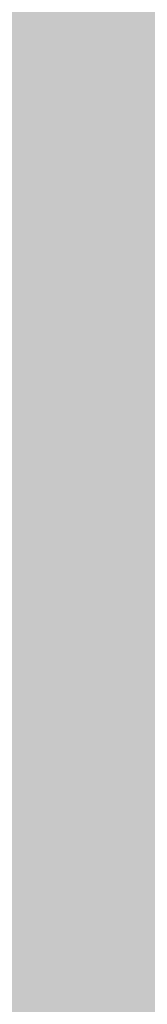
# Model space of a CAD drawing. Units: inches. Extents: x 2083 to 3317, y 1141 to 2115.
# Tile 227 of 256: x 3126.132 to 3126.67, y 1267.234 to 1271.372. Entities that reach past the tile are written whole.
import ezdxf

# ---------------------------------------------------------------- set-up
doc = ezdxf.new("R2010")
doc.units = ezdxf.units.IN
doc.layers.add('A-ANNO-DIMS', color=2, linetype='Continuous', lineweight=18)
doc.layers.add('A-WALL-PATT', color=251, linetype='Continuous', lineweight=13, true_color=0x636466)
doc.styles.get("Standard").update_dxf_attribs({"font": 'arial.ttf'})
doc.dimstyles.new('ISO-25', dxfattribs={"dimtxt": 12, "dimasz": 12, "dimexe": 1.25, "dimexo": 0.625, "dimtad": 1, "dimlunit": 3, "dimtxsty": 'Standard', "dimcen": 2.5, "dimadec": 0, "dimazin": 0, "dimtfac": 1, "dimtmove": 0, "dimatfit": 3, "dimfxl": 1, "dimarcsym": 0})

# ---------------------------------------------------------------- blocks, each defined once
blk = doc.blocks.new('*D26')
at = {"layer": 'A-ANNO-DIMS', "color": 0, "lineweight": -2, "transparency": 16777216}
for p, q in [((3088.9858, 1274.9151), (3088.9858, 1270.952)), ((3111.24, 1274.9151), (3111.24, 1270.952)), ((3076.9858, 1272.202), (2840.2624, 1272.202)), ((3111.24, 1272.202), (3088.9858, 1272.202)), ((3123.24, 1272.202), (3135.24, 1272.202))]:
    blk.add_line(p, q, dxfattribs=at)
at = {"layer": 'A-ANNO-DIMS', "color": 0, "transparency": 16777216}
for points in [[(3076.9858, 1274.202), (3076.9858, 1270.202), (3088.9858, 1272.202)], [(3123.24, 1274.202), (3123.24, 1270.202), (3111.24, 1272.202)]]:
    blk.add_solid(points, dxfattribs=at)
at = {"layer": 'Defpoints', "color": 0, "transparency": 16777216}
for p in [(3088.9858, 1275.5401), (3111.24, 1275.5401), (3088.9858, 1272.202)]:
    blk.add_point(p, dxfattribs=at)
at = {"layer": 'A-ANNO-DIMS', "color": 0, "transparency": 16777216, "insert": (2952.6241, 1279.0316), "char_height": 12, "attachment_point": 5}
blk.add_mtext('NIGHTSTAND 1\'-10 1/2" TYP.', dxfattribs=at)
blk = doc.blocks.new('*D27')
at = {"layer": 'A-ANNO-DIMS', "color": 0, "lineweight": -2, "transparency": 16777216}
for p, q in [((3114.5782, 1309.7943), (3114.5782, 1321.7943)), ((3111.865, 1297.7943), (3115.8282, 1297.7943)), ((3114.5782, 1297.7943), (3114.5782, 1275.5401)), ((3111.865, 1275.5401), (3115.8282, 1275.5401)), ((3114.5782, 1263.5401), (3114.5782, 1140.9886))]:
    blk.add_line(p, q, dxfattribs=at)
at = {"layer": 'A-ANNO-DIMS', "color": 0, "transparency": 16777216}
for points in [[(3112.5782, 1309.7943), (3116.5782, 1309.7943), (3114.5782, 1297.7943)], [(3112.5782, 1263.5401), (3116.5782, 1263.5401), (3114.5782, 1275.5401)]]:
    blk.add_solid(points, dxfattribs=at)
at = {"layer": 'Defpoints', "color": 0, "transparency": 16777216}
for p in [(3111.24, 1297.7943), (3111.24, 1275.5401), (3114.5782, 1275.5401)]:
    blk.add_point(p, dxfattribs=at)
at = {"layer": 'A-ANNO-DIMS', "color": 0, "transparency": 16777216, "insert": (3107.7485, 1196.2643), "char_height": 12, "attachment_point": 5, "rotation": 90}
blk.add_mtext('1\'-10 1/2" TYP.', dxfattribs=at)

msp = doc.modelspace()

# ---------------------------------------------------------------- hatches: boundary and pattern name
at = {"layer": 'A-WALL-PATT'}
h = msp.add_hatch(color=256, dxfattribs=at)
h.dxf.hatch_style = 1
h.paths.add_polyline_path([(3126.9598, 2020.7614), (2748.9598, 2020.7614), (2604.9598, 2020.7614), (2226.9598, 2020.7614), (2226.9598, 1702.7614), (2466.9598, 1702.7614), (2466.9598, 1582.7614), (2418.9598, 1582.7614), (2418.9598, 1477.7614), (2226.9598, 1477.7614), (2226.9598, 1263.2614), (2544.9598, 1263.2614), (2544.9598, 1411.7614), (2604.9598, 1411.7614), (2685.9598, 1411.7614), (2685.9598, 1420.7614), (2604.9598, 1420.7614), (2604.9598, 1573.7614), (2604.9598, 1702.7614), (2604.9598, 2011.7614), (2748.9598, 2011.7614), (2748.9598, 1702.7614), (2862.9598, 1702.7614), (2862.9598, 1621.7614), (2871.9598, 1621.7614), (2871.9598, 1702.7614), (2883.9598, 1702.7614), (2883.9598, 1706.9395, -0.026459), (2883.9598, 1711.7614), (2757.9598, 1711.7614), (2757.9598, 1807.7614), (2787.9598, 1807.7614), (2787.9598, 1812.2614), (2757.9598, 1812.2614), (2757.9598, 2011.7614), (2877.9598, 2011.7614), (2877.9598, 1812.2614), (2847.9598, 1812.2614), (2847.9598, 1807.7614), (2889.8357, 1807.7614), (2889.8357, 1812.2614), (2882.4598, 1812.2614), (2882.4598, 2011.7614), (3117.9598, 2011.7614), (3117.9598, 1812.2614), (2937.8357, 1812.2614), (2937.8357, 1807.7614), (2995.7098, 1807.7614), (2995.7098, 1796.1177), (3000.2098, 1796.1177), (3000.2098, 1807.7614), (3117.9598, 1807.7614), (3117.9598, 1711.7614), (3000.2098, 1711.7614), (3000.2098, 1760.1177), (2998.5727, 1760.1177, -0.020711), (2995.7098, 1760.1177), (2995.7098, 1711.7614), (2931.9598, 1711.7614), (2931.9598, 1702.7614), (3126.9598, 1702.7614)])
h.paths.add_polyline_path([(2471.4598, 2011.7614), (2471.4598, 1810.0114), (2462.7169, 1810.0114), (2462.7169, 1805.5114), (2505.9598, 1805.5114), (2505.9598, 1810.0114), (2475.9598, 1810.0114), (2475.9598, 2011.7614), (2595.9598, 2011.7614), (2595.9598, 1810.0114), (2565.9598, 1810.0114), (2565.9598, 1805.5114), (2595.9598, 1805.5114), (2595.9598, 1711.7614), (2235.9598, 1711.7614), (2235.9598, 1805.5114), (2353.7098, 1805.5114), (2353.7098, 1796.0542), (2358.2098, 1796.0542), (2358.2098, 1805.5114), (2414.7169, 1805.5114), (2414.7169, 1810.0114), (2235.9598, 1810.0114), (2235.9598, 2011.7614)], flags=16)
h.paths.add_polyline_path([(2270.2047, 1994.61), (2270.2047, 1970.61), (2246.2047, 1970.61), (2246.2047, 1994.61)], flags=0)
edge = h.paths.add_edge_path(flags=0)
edge.add_ellipse((2332.0274, 1899.7982), major_axis=(-3.043, 3.043), ratio=0.168252, start_angle=-161.3322, end_angle=-156.3071, ccw=False)
edge.add_ellipse((2333.082, 1898.7435), major_axis=(-1.0546, 1.0546), ratio=0.453532, start_angle=-123.371, end_angle=-94.1591)
edge = h.paths.add_edge_path(flags=0)
edge.add_ellipse((2332.0274, 1968.8763), major_axis=(3.043, 3.043), ratio=0.168252, start_angle=18.6678, end_angle=23.6929)
edge.add_spline(control_points=[(2332.9256, 1970.6911), (2332.2268, 1970.3361), (2330.8937, 1969.6589), (2328.4131, 1970.9321), (2327.2039, 1967.7487), (2324.7096, 1969.9556), (2322.5328, 1967.0124), (2320.0128, 1971.2958), (2317.6803, 1968.1578), (2316.0405, 1967.102), (2315.4269, 1966.8096)], knot_values=[0, 0, 0, 0, 2.267059, 4.324559, 6.685584, 8.878641, 11.121502, 14.300359, 17.755284, 19.732645, 19.732645, 19.732645, 19.732645], degree=3, periodic=0)
edge.add_ellipse((2332.0274, 1968.8763), major_axis=(3.043, 3.043), ratio=0.168252, start_angle=18.6678, end_angle=23.6929, ccw=False)
edge.add_ellipse((2333.082, 1969.9309), major_axis=(1.0546, 1.0546), ratio=0.453532, start_angle=56.629, end_angle=85.8409, ccw=False)
edge = h.paths.add_edge_path(flags=0)
edge.add_spline(control_points=[(2296.4283, 1967.9879), (2293.6278, 1965.3363), (2287.7036, 1959.7271), (2299.7439, 1949.9957), (2294.5326, 1935.6685), (2290.5732, 1920.6035), (2293.3941, 1909.9737), (2296.1854, 1904.9665)], knot_values=[0.099185, 0.099185, 0.099185, 0.099185, 0.345301, 0.619822, 0.982653, 1.386093, 1.810555, 1.810555, 1.810555, 1.810555], degree=3, periodic=0)
edge.add_spline(control_points=[(2296.1854, 1904.9665), (2297.3836, 1902.6193), (2298.001, 1901.9493), (2298.553, 1901.4682)], knot_values=[0.006246, 0.006246, 0.006246, 0.006246, 0.055476, 0.055476, 0.055476, 0.055476], degree=3, periodic=0)
edge.add_spline(control_points=[(2298.553, 1901.4682), (2297.2586, 1900.9232), (2295.2253, 1900.2321), (2293.0602, 1900.6142), (2292.1014, 1900.7884), (2292.0896, 1900.7906)], knot_values=[0.312835, 0.312835, 0.312835, 0.312835, 0.40178, 0.474987, 0.475903, 0.475903, 0.475903, 0.475903], degree=3, periodic=0)
edge.add_arc((2292.7936, 1904.6641), 3.937, 215.4209, 259.6982, ccw=False)
edge.add_spline(control_points=[(2289.5853, 1902.3823), (2289.4767, 1902.5351), (2289.3685, 1902.688), (2289.2609, 1902.8412)], knot_values=[0.102872, 0.102872, 0.102872, 0.102872, 0.116896, 0.116896, 0.116896, 0.116896], degree=3, periodic=0)
edge.add_spline(control_points=[(2289.2609, 1902.8412), (2288.6866, 1902.5502), (2287.64, 1902.0199), (2285.8813, 1901.874), (2283.853, 1901.5044), (2281.72, 1899.7105), (2278.467, 1899.4929), (2276.1571, 1901.8832), (2272.259, 1899.8041), (2267.7776, 1901.8432), (2262.2439, 1900.184), (2257.4149, 1901.7821), (2254.3184, 1900.7261), (2253.1783, 1900.3373)], knot_values=[0, 0, 0, 0, 1.907977, 3.477176, 5.261074, 7.972851, 11.680248, 13.717921, 16.939592, 22.789562, 27.502503, 33.595215, 37.145618, 37.145618, 37.145618, 37.145618], degree=3, periodic=0)
edge.add_line((2253.1783, 1900.3373), (2250.2442, 1902.8412))
edge.add_line((2250.2442, 1902.8412), (2250.2442, 1965.8333))
edge.add_line((2250.2442, 1965.8333), (2253.1783, 1968.3371))
edge.add_spline(control_points=[(2253.1783, 1968.3371), (2254.3184, 1967.9483), (2257.4149, 1966.8924), (2262.2439, 1968.4904), (2267.7776, 1966.8313), (2271.5267, 1968.5372), (2273.8759, 1967.8283), (2274.2067, 1967.7276)], knot_values=[0, 0, 0, 0, 0.09018, 0.244935, 0.364644, 0.513233, 0.537855, 0.537855, 0.537855, 0.537855], degree=3, periodic=0)
edge.add_arc((2274.3529, 1963.7933), 3.937, 72.0511, 92.1279, ccw=False)
edge.add_arc((2281.2969, 1985.23), 18.5963, 252.05113, 288.56572)
edge.add_arc((2292.3167, 1956.0289), 12.6461, 71.02679, 113.77822, ccw=False)
edge = h.paths.add_edge_path(flags=0)
edge.add_spline(control_points=[(2274.8994, 1951.8562), (2275.0662, 1951.6166), (2275.2327, 1951.3766), (2275.398, 1951.1359)], knot_values=[1.409916, 1.409916, 1.409916, 1.409916, 1.43159, 1.43159, 1.43159, 1.43159], degree=3, periodic=0)
edge.add_spline(control_points=[(2275.398, 1951.1359), (2275.7921, 1950.5619), (2276.1792, 1949.9838), (2276.5455, 1949.3971)], knot_values=[1.358238, 1.358238, 1.358238, 1.358238, 1.409916, 1.409916, 1.409916, 1.409916], degree=3, periodic=0)
edge.add_line((2276.5455, 1949.3971), (2277.4373, 1947.8622))
edge.add_spline(control_points=[(2277.4373, 1947.8622), (2276.3038, 1945.6731), (2274.6397, 1942.4269), (2274.6316, 1938.0939), (2272.7991, 1930.8515), (2274.3564, 1943.897), (2275.9477, 1947.9234), (2276.5455, 1949.3971)], knot_values=[0.005632, 0.005632, 0.005632, 0.005632, 0.186014, 0.266002, 0.357087, 0.59639, 0.739732, 0.739732, 0.739732, 0.739732], degree=3, periodic=0)
edge.add_spline(control_points=[(2276.5455, 1949.3971), (2276.1792, 1949.9838), (2275.7921, 1950.5619), (2275.398, 1951.1359)], knot_values=[1.358238, 1.358238, 1.358238, 1.358238, 1.409916, 1.409916, 1.409916, 1.409916], degree=3, periodic=0)
edge.add_spline(control_points=[(2275.398, 1951.1359), (2274.9425, 1950.0805), (2274.2078, 1948.0253), (2273.9346, 1944.8515), (2272.4685, 1937.6275), (2273.4662, 1945.6965), (2274.7006, 1951.0595), (2274.8994, 1951.8562)], knot_values=[0.104364, 0.104364, 0.104364, 0.104364, 0.189636, 0.269624, 0.36071, 0.600013, 0.644622, 0.644622, 0.644622, 0.644622], degree=3, periodic=0)
h.paths.add_polyline_path([(2269.1675, 1963.1276, -0.357527), (2268.1706, 1960.9764, -0.092561), (2268.1706, 1939.4363, -0.357527), (2269.1675, 1937.2851, -0.357527), (2267.0163, 1938.282, -0.164785), (2254.6856, 1938.282, -0.357527), (2252.5344, 1937.2851, -0.357527), (2253.5313, 1939.4363, -0.092561), (2253.5313, 1960.9764, -0.357527), (2252.5344, 1963.1276, -0.357527), (2254.6856, 1962.1307, -0.164785), (2267.0163, 1962.1307, -0.357527)], flags=0)
h.paths.add_polyline_path([(2248.8741, 1967.8018), (2248.8741, 1957.0277), (2249.4578, 1957.0277), (2249.4578, 1911.6468), (2248.8741, 1911.6468), (2248.8741, 1900.8727), (2246.5119, 1900.8727, 0.197327), (2244.1497, 1902.4569), (2244.1497, 1966.2176, 0.197327), (2246.5119, 1967.8018)], flags=0)
h.paths.add_polyline_path([(2269.1675, 1931.3893, -0.357527), (2268.1706, 1929.2381, -0.092561), (2268.1706, 1907.6981, -0.357527), (2269.1675, 1905.5469, -0.357527), (2267.0163, 1906.5438, -0.164785), (2254.6856, 1906.5438, -0.357527), (2252.5344, 1905.5469, -0.357527), (2253.5313, 1907.6981, -0.092561), (2253.5313, 1929.2381, -0.357527), (2252.5344, 1931.3893, -0.357527), (2254.6856, 1930.3925, -0.164785), (2267.0163, 1930.3925, -0.357527)], flags=0)
edge = h.paths.add_edge_path(flags=0)
edge.add_spline(control_points=[(2276.1969, 1906.7237), (2276.1681, 1909.0289), (2276.114, 1913.3719), (2270.5984, 1924.925), (2273.9052, 1919.0128), (2275.9217, 1916.2621), (2275.4746, 1912.4021), (2277.2579, 1910.3806), (2276.696, 1908.225), (2276.6462, 1906.813), (2276.6178, 1906.0084)], knot_values=[0, 0, 0, 0, 8.61026, 16.221274, 18.843057, 23.804898, 27.440828, 29.356102, 31.203478, 33.650687, 33.650687, 33.650687, 33.650687], degree=3, periodic=0)
edge.add_spline(control_points=[(2276.6178, 1906.0084), (2276.6233, 1905.6241), (2276.4977, 1904.6287), (2275.4418, 1903.8547), (2274.9373, 1903.0804), (2274.8591, 1902.8412)], knot_values=[0.156488, 0.156488, 0.156488, 0.156488, 0.184398, 0.231376, 0.250598, 0.250598, 0.250598, 0.250598], degree=3, periodic=0)
edge.add_line((2274.8591, 1902.8412), (2276.506, 1902.8412))
edge.add_spline(control_points=[(2276.506, 1902.8412), (2276.7883, 1903.0849), (2277.6651, 1904.1252), (2278.2495, 1904.3407), (2277.6539, 1908.5274), (2278.1557, 1906.2278), (2278.1005, 1905.2859), (2278.8467, 1904.069), (2277.8568, 1903.4149), (2277.8742, 1902.991), (2277.9036, 1902.8412)], knot_values=[0.059574, 0.059574, 0.059574, 0.059574, 0.080753, 0.103741, 0.16972, 0.176036, 0.207137, 0.240474, 0.262341, 0.27366, 0.27366, 0.27366, 0.27366], degree=3, periodic=0)
edge.add_line((2277.9036, 1902.8412), (2280.0298, 1902.8412))
edge.add_spline(control_points=[(2280.0298, 1902.8412), (2279.8882, 1903.0884), (2279.4993, 1903.9816), (2280.1523, 1905.9393), (2278.1036, 1909.6578), (2279.7624, 1907.1853), (2280.3279, 1904.8749), (2280.4851, 1903.4896), (2281.4633, 1903.2494), (2281.7583, 1902.9365), (2281.834, 1902.8412)], knot_values=[0.013856, 0.013856, 0.013856, 0.013856, 0.034874, 0.088867, 0.107879, 0.126738, 0.158714, 0.193757, 0.217487, 0.226722, 0.226722, 0.226722, 0.226722], degree=3, periodic=0)
edge.add_spline(control_points=[(2281.834, 1902.8412), (2281.7875, 1902.8267), (2281.647, 1902.783), (2281.3955, 1902.8595), (2281.0881, 1902.9852), (2280.7207, 1903.0609), (2280.3335, 1903.0257), (2280.1248, 1902.8989), (2280.0298, 1902.8412)], knot_values=[0, 0, 0, 0, 0.14413, 0.435517, 0.749276, 1.153046, 1.548371, 1.878348, 1.878348, 1.878348, 1.878348], degree=3, periodic=0)
edge.add_line((2280.0298, 1902.8412), (2277.9036, 1902.8412))
edge.add_spline(control_points=[(2277.9036, 1902.8412), (2277.8929, 1902.7959), (2277.8654, 1902.6796), (2277.6075, 1902.6875), (2277.2741, 1902.8007), (2276.8379, 1902.6198), (2276.5838, 1902.7893), (2276.506, 1902.8412)], knot_values=[0, 0, 0, 0, 0.127189, 0.326199, 0.628009, 1.24357, 1.515331, 1.515331, 1.515331, 1.515331], degree=3, periodic=0)
edge.add_line((2276.506, 1902.8412), (2274.8591, 1902.8412))
edge.add_spline(control_points=[(2274.8591, 1902.8412), (2274.8144, 1902.8986), (2274.7251, 1903.0134), (2274.4935, 1903.119), (2274.2443, 1902.9605), (2273.9371, 1903.1849), (2273.614, 1902.9831), (2273.4083, 1902.883), (2273.3223, 1902.8412)], knot_values=[0, 0, 0, 0, 0.21843, 0.436957, 0.687977, 0.990379, 1.398396, 1.69185, 1.69185, 1.69185, 1.69185], degree=3, periodic=0)
edge.add_spline(control_points=[(2273.3223, 1902.8412), (2273.6167, 1903.4457), (2274.274, 1904.5383), (2276.0272, 1904.5737), (2276.207, 1906.5836), (2276.1969, 1906.7237)], knot_values=[0.012227, 0.012227, 0.012227, 0.012227, 0.059472, 0.106218, 0.134458, 0.134458, 0.134458, 0.134458], degree=3, periodic=0)
h.paths.add_polyline_path([(2270.7761, 1897.7898), (2270.7761, 1873.7898), (2246.7761, 1873.7898), (2246.7761, 1897.7898)], flags=0)
h.paths.add_polyline_path([(2353.7098, 1760.0051), (2353.7098, 1760.0542), (2358.2098, 1760.0542, -0.033729)], flags=0)
h.paths.add_polyline_path([(2321.8191, 1737.5292), (2341.9953, 1737.5292, -0.414214), (2343.2033, 1736.3212), (2343.2033, 1721.0206, -0.414214), (2341.9953, 1719.8127), (2321.8191, 1719.8127, -0.414214), (2320.6112, 1721.0206), (2320.6112, 1736.3212, -0.414214)], flags=0)
h.paths.add_polyline_path([(2324.235, 1736.3212), (2339.5794, 1736.3212, -0.414214), (2341.9953, 1733.9053), (2341.9953, 1725.4497, -0.414214), (2339.5794, 1723.0338), (2333.6806, 1723.0338), (2333.8453, 1722.0455, -0.870646), (2335.4254, 1721.8259, -0.767327), (2333.9227, 1721.4232), (2331.291, 1721.4232, -0.767327), (2329.7883, 1721.8259, -0.870646), (2331.3684, 1722.0455), (2331.5331, 1723.0338), (2324.235, 1723.0338, -0.414214), (2321.8191, 1725.4497), (2321.8191, 1733.9053, -0.414214)], flags=0)
h.paths.add_polyline_path([(2570.4838, 1928.6154), (2589.6838, 1928.6154), (2590.1688, 1928.6154), (2590.1688, 1904.9934), (2570.4838, 1904.9934)], flags=0)
h.paths.add_polyline_path([(2574.4473, 1927.2638, -1), (2572.8288, 1927.2638, -1)], flags=0)
h.paths.add_polyline_path([(2573.0899, 1926.9409), (2573.925, 1927.776), (2574.1477, 1927.5533), (2573.3126, 1926.7182)], flags=0)
h.paths.add_polyline_path([(2578.7791, 1919.7296, -1), (2571.5917, 1919.7296, -1)], flags=0)
h.paths.add_polyline_path([(2578.3854, 1919.7296, -1), (2571.9854, 1919.7296, -1)], flags=0)
h.paths.add_polyline_path([(2331.5958, 1729.4762, -1), (2333.618, 1729.4762, -1)], flags=0)
h.paths.add_polyline_path([(2578.0342, 1927.2638, -1), (2576.4157, 1927.2638, -1)], flags=0)
h.paths.add_polyline_path([(2576.6889, 1927.5311), (2576.9116, 1927.7538), (2577.7467, 1926.9186), (2577.524, 1926.6959)], flags=0)
h.paths.add_polyline_path([(2578.1391, 1909.8595, -1), (2572.2317, 1909.8595, -1)], flags=0)
h.paths.add_polyline_path([(2577.7454, 1909.8595, -1), (2572.6254, 1909.8595, -1)], flags=0)
h.paths.add_polyline_path([(2583.7977, 1927.2638, -1), (2582.1792, 1927.2638, -1)], flags=0)
h.paths.add_polyline_path([(2582.7186, 1927.7538), (2583.5538, 1926.9186), (2583.3311, 1926.6959), (2582.4959, 1927.5311)], flags=0)
h.paths.add_polyline_path([(2582.4959, 1927.5311), (2582.7186, 1927.7538), (2583.5538, 1926.9186), (2583.3311, 1926.6959)], flags=0)
h.paths.add_polyline_path([(2587.7391, 1920.5296, -1), (2581.8317, 1920.5296, -1)], flags=0)
h.paths.add_polyline_path([(2587.3454, 1920.5296, -1), (2582.2254, 1920.5296, -1)], flags=0)
h.paths.add_polyline_path([(2587.3846, 1927.2638, -1), (2585.7661, 1927.2638, -1)], flags=0)
h.paths.add_polyline_path([(2586.082, 1926.9802), (2586.9172, 1927.8154), (2587.1399, 1927.5927), (2586.3047, 1926.7575)], flags=0)
h.paths.add_polyline_path([(2588.3791, 1910.6595, -1), (2581.1917, 1910.6595, -1)], flags=0)
h.paths.add_polyline_path([(2587.9854, 1910.6595, -1), (2581.5854, 1910.6595, -1)], flags=0)
h.paths.add_polyline_path([(2417.1677, 1729.4779), (2437.3439, 1729.4779, -0.414214), (2438.5519, 1728.2699), (2438.5519, 1712.9693, -0.414214), (2437.3439, 1711.7614), (2417.1677, 1711.7614, -0.414214), (2415.9598, 1712.9693), (2415.9598, 1728.2699, -0.414214)], flags=0)
h.paths.add_polyline_path([(2419.5836, 1728.2699), (2434.928, 1728.2699, -0.414214), (2437.3439, 1725.8541), (2437.3439, 1717.3984, -0.414214), (2434.928, 1714.9825), (2429.0292, 1714.9825), (2429.1939, 1713.9942, -0.870646), (2430.774, 1713.7746, -0.767327), (2429.2713, 1713.372), (2426.6396, 1713.372, -0.767327), (2425.1369, 1713.7746, -0.870646), (2426.717, 1713.9942), (2426.8817, 1714.9825), (2419.5836, 1714.9825, -0.414214), (2417.1677, 1717.3984), (2417.1677, 1725.8541, -0.414214)], flags=0)
h.paths.add_polyline_path([(2419.5836, 1728.2699), (2434.928, 1728.2699, -0.414214), (2437.3439, 1725.8541), (2437.3439, 1717.3984, -0.414214), (2434.928, 1714.9825), (2429.0292, 1714.9825), (2428.3581, 1719.009), (2427.5528, 1719.009), (2426.8817, 1714.9825), (2419.5836, 1714.9825, -0.414214), (2417.1677, 1717.3984), (2417.1677, 1725.8541, -0.414214)], flags=0)
h.paths.add_polyline_path([(2426.9444, 1721.4249, -1), (2428.9666, 1721.4249, -1)], flags=0)
h.paths.add_polyline_path([(2475.9598, 1702.7614), (2595.9598, 1702.7614), (2595.9598, 1582.7614), (2475.9598, 1582.7614)], flags=16)
h.paths.add_polyline_path([(2427.9598, 1573.7614), (2595.9598, 1573.7614), (2595.9598, 1468.7614), (2595.9598, 1420.7614), (2384.4598, 1420.7614), (2384.4598, 1468.7614), (2427.9598, 1468.7614)], flags=16)
h.paths.add_polyline_path([(2379.9598, 1468.7614), (2379.9598, 1420.7614), (2235.9598, 1420.7614), (2235.9598, 1468.7614)], flags=16)
h.paths.add_polyline_path([(2317.816, 1466.6958), (2337.9922, 1466.6958, -0.414214), (2339.2002, 1465.4878), (2339.2002, 1450.1872, -0.414214), (2337.9922, 1448.9792), (2317.816, 1448.9792, -0.414214), (2316.6081, 1450.1872), (2316.6081, 1465.4878, -0.414214)], flags=0)
h.paths.add_polyline_path([(2320.2319, 1465.4878), (2335.5763, 1465.4878, -0.414214), (2337.9922, 1463.0719), (2337.9922, 1454.6163, -0.414214), (2335.5763, 1452.2004), (2329.6775, 1452.2004), (2329.8422, 1451.212, -0.870646), (2331.4223, 1450.9925, -0.767327), (2329.9196, 1450.5898), (2327.2879, 1450.5898, -0.767327), (2325.7852, 1450.9925, -0.870646), (2327.3653, 1451.212), (2327.53, 1452.2004), (2320.2319, 1452.2004, -0.414214), (2317.816, 1454.6163), (2317.816, 1463.0719, -0.414214)], flags=0)
h.paths.add_polyline_path([(2320.2319, 1465.4878), (2335.5763, 1465.4878, -0.414214), (2337.9922, 1463.0719), (2337.9922, 1454.6163, -0.414214), (2335.5763, 1452.2004), (2329.6775, 1452.2004), (2329.0064, 1456.2269), (2328.2011, 1456.2269), (2327.53, 1452.2004), (2320.2319, 1452.2004, -0.414214), (2317.816, 1454.6163), (2317.816, 1463.0719, -0.414214)], flags=0)
h.paths.add_polyline_path([(2327.5926, 1458.6428, -1), (2329.6148, 1458.6428, -1)], flags=0)
h.paths.add_polyline_path([(2244.4117, 1433.3405), (2241.9209, 1433.3405, -0.414214), (2240.0179, 1435.2435), (2240.0179, 1440.9528, -0.414211), (2241.9209, 1442.8559), (2244.4117, 1442.8559, -1.976472)], flags=0)
h.paths.add_polyline_path([(2245.3569, 1434.3975, -0.414214), (2245.3569, 1441.7988, -2.144098)], flags=0)
h.paths.add_polyline_path([(2535.9598, 1416.2614), (2535.9598, 1272.2614), (2235.9598, 1272.2614), (2235.9598, 1416.2614)], flags=16)
h.paths.add_polyline_path([(2260.1196, 1384.2928), (2260.1196, 1362.0386), (2237.8654, 1362.0386), (2237.8654, 1384.2928)], flags=0)
edge = h.paths.add_edge_path(flags=0)
edge.add_line((2318.2518, 1362.0933), (2318.1458, 1362.001))
edge.add_ellipse((2317.4451, 1360.431), major_axis=(2.8216, 2.8216), ratio=0.168252, start_angle=18.6678, end_angle=20.9481, ccw=False)
edge.add_ellipse((2318.423, 1361.409), major_axis=(0.9779, 0.9779), ratio=0.453532, start_angle=56.629, end_angle=70.2262, ccw=False)
edge = h.paths.add_edge_path(flags=0)
edge.add_line((2319.1074, 1295.5711), (2319.015, 1295.6771))
edge.add_ellipse((2317.4451, 1296.3778), major_axis=(-2.8216, 2.8216), ratio=0.168252, start_angle=-161.3322, end_angle=-159.0519, ccw=False)
edge.add_ellipse((2318.423, 1295.3999), major_axis=(-0.9779, 0.9779), ratio=0.453532, start_angle=-123.371, end_angle=-109.7738)
edge = h.paths.add_edge_path(flags=0)
edge.add_spline(control_points=[(2284.2103, 1301.1702), (2284.5807, 1300.4447), (2284.8912, 1299.892), (2285.1596, 1299.461)], knot_values=[0.039066, 0.039066, 0.039066, 0.039066, 0.055476, 0.055476, 0.055476, 0.055476], degree=3, periodic=0)
edge.add_line((2285.1596, 1299.461), (2284.2103, 1301.1702))
edge = h.paths.add_edge_path(flags=0)
edge.add_line((2280.4125, 1297.298), (2283.37, 1297.0361))
edge.add_line((2283.37, 1297.0361), (2286.4057, 1297.9263))
edge.add_spline(control_points=[(2286.4057, 1297.9263), (2285.3055, 1297.4631), (2284.3448, 1297.1292), (2283.37, 1297.0361)], knot_values=[0.394369, 0.394369, 0.394369, 0.394369, 0.475903, 0.475903, 0.475903, 0.475903], degree=3, periodic=0)
edge.add_spline(control_points=[(2283.37, 1297.0361), (2283.2814, 1297.0277), (2282.3163, 1296.9573), (2281.3125, 1297.1345), (2280.4234, 1297.296), (2280.4125, 1297.298)], knot_values=[0.312835, 0.312835, 0.312835, 0.312835, 0.320246, 0.393453, 0.394369, 0.394369, 0.394369, 0.394369], degree=3, periodic=0)
edge = h.paths.add_edge_path(flags=0)
edge.add_line((2284.4356, 1359.6073), (2280.4463, 1355.328))
edge.add_line((2280.4463, 1355.328), (2279.58, 1351.0178))
edge.add_line((2279.58, 1351.0178), (2282.413, 1346.5804))
edge.add_spline(control_points=[(2282.413, 1346.5804), (2283.1533, 1345.5892), (2284.2529, 1344.0289), (2284.801, 1342.3872), (2284.9352, 1341.8055)], knot_values=[1.240098, 1.240098, 1.240098, 1.240098, 1.332892, 1.382712, 1.382712, 1.382712, 1.382712], degree=3, periodic=0)
edge.add_spline(control_points=[(2284.9352, 1341.8055), (2285.3191, 1340.1406), (2285.233, 1338.4092), (2284.9099, 1336.6541)], knot_values=[1.097484, 1.097484, 1.097484, 1.097484, 1.240098, 1.240098, 1.240098, 1.240098], degree=3, periodic=0)
edge.add_spline(control_points=[(2284.9099, 1336.6541), (2284.5868, 1334.899), (2284.0267, 1333.1203), (2283.4626, 1331.3606)], knot_values=[0.95487, 0.95487, 0.95487, 0.95487, 1.097484, 1.097484, 1.097484, 1.097484], degree=3, periodic=0)
edge.add_line((2283.4626, 1331.3606), (2281.8904, 1326.1534))
edge.add_line((2281.8904, 1326.1534), (2280.7563, 1321.0561))
edge.add_line((2280.7563, 1321.0561), (2280.2992, 1316.002))
edge.add_line((2280.2992, 1316.002), (2280.7159, 1310.9501))
edge.add_line((2280.7159, 1310.9501), (2282.0281, 1305.9721))
edge.add_line((2282.0281, 1305.9721), (2284.2103, 1301.1702))
edge.add_spline(control_points=[(2284.2103, 1301.1702), (2283.3407, 1302.7302), (2282.6119, 1304.3365), (2282.0281, 1305.9721)], knot_values=[0.099185, 0.099185, 0.099185, 0.099185, 0.241799, 0.241799, 0.241799, 0.241799], degree=3, periodic=0)
edge.add_spline(control_points=[(2282.0281, 1305.9721), (2281.4443, 1307.6078), (2281.0055, 1309.2728), (2280.7159, 1310.9501)], knot_values=[0.241799, 0.241799, 0.241799, 0.241799, 0.384413, 0.384413, 0.384413, 0.384413], degree=3, periodic=0)
edge.add_spline(control_points=[(2280.7159, 1310.9501), (2280.4332, 1312.5876), (2280.2894, 1314.277), (2280.2989, 1315.962), (2280.2992, 1316.002)], knot_values=[0.384413, 0.384413, 0.384413, 0.384413, 0.523647, 0.527028, 0.527028, 0.527028, 0.527028], degree=3, periodic=0)
edge.add_spline(control_points=[(2280.2992, 1316.002), (2280.3123, 1317.687), (2280.4779, 1319.3679), (2280.7563, 1321.0561)], knot_values=[0.527028, 0.527028, 0.527028, 0.527028, 0.669642, 0.669642, 0.669642, 0.669642], degree=3, periodic=0)
edge.add_spline(control_points=[(2280.7563, 1321.0561), (2281.0346, 1322.7443), (2281.4259, 1324.4396), (2281.8904, 1326.1534)], knot_values=[0.669642, 0.669642, 0.669642, 0.669642, 0.812256, 0.812256, 0.812256, 0.812256], degree=3, periodic=0)
edge.add_spline(control_points=[(2281.8904, 1326.1534), (2282.2644, 1327.5333), (2282.7879, 1329.2618), (2283.3528, 1331.0178), (2283.4626, 1331.3606)], knot_values=[0.812256, 0.812256, 0.812256, 0.812256, 0.927087, 0.95487, 0.95487, 0.95487, 0.95487], degree=3, periodic=0)
edge.add_line((2283.4626, 1331.3606), (2284.9099, 1336.6541))
edge.add_line((2284.9099, 1336.6541), (2284.9352, 1341.8055))
edge.add_line((2284.9352, 1341.8055), (2282.413, 1346.5804))
edge.add_spline(control_points=[(2282.413, 1346.5804), (2281.2751, 1348.1038), (2280.0784, 1349.5703), (2279.58, 1351.0178)], knot_values=[1.382712, 1.382712, 1.382712, 1.382712, 1.525326, 1.525326, 1.525326, 1.525326], degree=3, periodic=0)
edge.add_spline(control_points=[(2279.58, 1351.0178), (2279.4433, 1351.4147), (2279.1363, 1352.8569), (2279.7352, 1354.2904), (2280.4463, 1355.328)], knot_values=[1.525326, 1.525326, 1.525326, 1.525326, 1.564439, 1.667941, 1.667941, 1.667941, 1.667941], degree=3, periodic=0)
edge.add_spline(control_points=[(2280.4463, 1355.328), (2281.4261, 1356.7578), (2282.9308, 1358.1826), (2284.4356, 1359.6073)], knot_values=[1.667941, 1.667941, 1.667941, 1.667941, 1.810555, 1.810555, 1.810555, 1.810555], degree=3, periodic=0)
edge.add_arc((2280.6231, 1348.5182), 11.7262, 71.02679, 113.77822)
edge.add_arc((2270.4049, 1375.5952), 17.2436, 252.05113, 288.56572, ccw=False)
edge.add_arc((2263.966, 1355.7178), 3.6506, 72.0511, 92.1279)
edge.add_arc((2263.966, 1355.7178), 3.6506, 92.1279, 177.9851)
edge.add_spline(control_points=[(2260.3176, 1355.8462), (2260.2604, 1354.2207), (2260.5513, 1350.1865), (2262.9993, 1346.7663), (2264.4727, 1344.649)], knot_values=[1.43159, 1.43159, 1.43159, 1.43159, 1.564144, 1.770695, 1.770695, 1.770695, 1.770695], degree=3, periodic=0)
edge.add_line((2264.4727, 1344.649), (2264.9356, 1343.9825))
edge.add_spline(control_points=[(2263.801, 1340.2481), (2263.8432, 1340.5141), (2264.0672, 1341.7565), (2264.5127, 1343.0025), (2264.935, 1343.9811)], knot_values=[0.53657, 0.53657, 0.53657, 0.53657, 0.559349, 0.644622, 0.644622, 0.644622, 0.644622], degree=3, periodic=0)
edge.add_spline(control_points=[(2264.935, 1343.9811), (2265.1178, 1343.715), (2265.2989, 1343.4479), (2265.4768, 1343.1794)], knot_values=[1.384077, 1.384077, 1.384077, 1.384077, 1.409916, 1.409916, 1.409916, 1.409916], degree=3, periodic=0)
edge.add_spline(control_points=[(2265.4768, 1343.1794), (2265.6546, 1342.9108), (2265.8293, 1342.6408), (2265.9991, 1342.3688)], knot_values=[1.358238, 1.358238, 1.358238, 1.358238, 1.384077, 1.384077, 1.384077, 1.384077], degree=3, periodic=0)
edge.add_line((2265.9991, 1342.3688), (2266.826, 1340.9455))
edge.add_spline(control_points=[(2266.826, 1340.9455), (2268.8944, 1337.0897), (2271.3982, 1325.843), (2270.5162, 1310.5686), (2275.9194, 1301.8606), (2277.7895, 1299.1994)], knot_values=[0.116896, 0.116896, 0.116896, 0.116896, 0.472987, 1.050969, 1.313793, 1.313793, 1.313793, 1.313793], degree=3, periodic=0)
edge.add_spline(control_points=[(2277.7895, 1299.1994), (2277.8394, 1299.1285), (2277.8894, 1299.0575), (2277.9396, 1298.9866)], knot_values=[0.109884, 0.109884, 0.109884, 0.109884, 0.116896, 0.116896, 0.116896, 0.116896], degree=3, periodic=0)
edge.add_line((2277.9396, 1298.9866), (2277.7888, 1299.1991))
edge.add_spline(control_points=[(2277.7888, 1299.1991), (2277.2566, 1298.9294), (2276.2864, 1298.4379), (2275.0394, 1298.3344), (2274.3833, 1298.2389), (2274.2153, 1298.2093)], knot_values=[33.12187, 33.12187, 33.12187, 33.12187, 35.029056, 36.598255, 37.144827, 37.144827, 37.144827, 37.144827], degree=3, periodic=0)
edge.add_line((2274.2153, 1298.2093), (2273.0731, 1297.893))
edge.add_spline(control_points=[(2273.0731, 1297.893), (2272.3229, 1297.5798), (2271.0392, 1296.5105), (2269.2484, 1296.2261), (2268.4231, 1296.3747)], knot_values=[26.532584, 26.532584, 26.532584, 26.532584, 29.198919, 31.839101, 31.839101, 31.839101, 31.839101], degree=3, periodic=0)
edge.add_line((2268.4231, 1296.3747), (2263.8785, 1297.4575))
edge.add_spline(control_points=[(2263.8785, 1297.4575), (2263.5561, 1297.3594), (2261.8603, 1296.8387), (2260.2388, 1297.2824), (2258.9335, 1297.5165)], knot_values=[15.919551, 15.919551, 15.919551, 15.919551, 16.939592, 21.226067, 21.226067, 21.226067, 21.226067], degree=3, periodic=0)
edge.add_line((2258.9335, 1297.5165), (2254.0552, 1297.329))
edge.add_spline(control_points=[(2254.0552, 1297.329), (2253.7555, 1297.2958), (2252.1137, 1297.1652), (2250.4619, 1297.5442), (2249.1297, 1297.6679)], knot_values=[5.306517, 5.306517, 5.306517, 5.306517, 6.276435, 10.613034, 10.613034, 10.613034, 10.613034], degree=3, periodic=0)
edge.add_line((2249.1297, 1297.6679), (2244.3316, 1296.8778))
edge.add_line((2244.3316, 1296.8778), (2241.611, 1299.1994))
edge.add_line((2241.611, 1299.1994), (2241.611, 1357.6094))
edge.add_line((2241.611, 1357.6094), (2244.3316, 1359.9311))
edge.add_line((2244.3316, 1359.9311), (2252.7288, 1359.5427))
edge.add_spline(control_points=[(2252.7288, 1359.5427), (2252.8709, 1359.5464), (2253.3057, 1359.5482), (2253.7398, 1359.5143), (2254.0317, 1359.4824)], knot_values=[0.233291, 0.233291, 0.233291, 0.233291, 0.244935, 0.268927, 0.268927, 0.268927, 0.268927], degree=3, periodic=0)
edge.add_line((2254.0317, 1359.4824), (2259.5872, 1359.4164))
edge.add_spline(control_points=[(2259.5872, 1359.4164), (2260.6771, 1359.6285), (2262.0732, 1359.897), (2263.5237, 1359.4593), (2263.8304, 1359.366)], knot_values=[0.422516, 0.422516, 0.422516, 0.422516, 0.513233, 0.537855, 0.537855, 0.537855, 0.537855], degree=3, periodic=0)
edge.add_arc((2263.966, 1355.7178), 3.6506, 72.0511, 92.1279, ccw=False)
edge.add_arc((2270.4049, 1375.5952), 17.2436, 252.05113, 288.56572)
edge.add_arc((2280.6231, 1348.5182), 11.7262, 71.02679, 113.77822, ccw=False)
h.paths.add_polyline_path([(2240.3405, 1359.4347), (2240.3405, 1349.4444), (2240.8818, 1349.4444), (2240.8818, 1307.3645), (2240.3405, 1307.3645), (2240.3405, 1297.3741), (2238.1502, 1297.3741, 0.197327), (2235.9598, 1298.8431), (2235.9598, 1357.9657, 0.197327), (2238.1502, 1359.4347)], flags=0)
h.paths.add_polyline_path([(2259.1578, 1355.1005, -0.357527), (2258.2334, 1353.1058, -0.092561), (2258.2334, 1333.1326, -0.357527), (2259.1578, 1331.1379, -0.357527), (2257.1631, 1332.0622, -0.164785), (2245.7293, 1332.0622, -0.357527), (2243.7346, 1331.1379, -0.357527), (2244.6589, 1333.1326, -0.092561), (2244.6589, 1353.1058, -0.357527), (2243.7346, 1355.1005, -0.357527), (2245.7293, 1354.1761, -0.164785), (2257.1631, 1354.1761, -0.357527)], flags=0)
edge = h.paths.add_edge_path(flags=0)
edge.add_line((2265.9991, 1342.3688), (2266.826, 1340.9455))
edge.add_line((2266.826, 1340.9455), (2265.3076, 1337.8141))
edge.add_line((2265.3076, 1337.8141), (2264.3582, 1334.6529))
edge.add_line((2264.3582, 1334.6529), (2264.262, 1333.7997))
edge.add_spline(control_points=[(2264.262, 1333.7997), (2264.2084, 1333.1871), (2264.1621, 1332.3655), (2264.0071, 1331.4139), (2263.969, 1331.2018)], knot_values=[0.464444, 0.464444, 0.464444, 0.464444, 0.516691, 0.531608, 0.531608, 0.531608, 0.531608], degree=3, periodic=0)
edge.add_spline(control_points=[(2263.969, 1331.2018), (2263.7745, 1330.1189), (2263.4244, 1328.7908), (2263.2574, 1328.5307), (2263.234, 1328.5146)], knot_values=[0.372682, 0.372682, 0.372682, 0.372682, 0.44885, 0.464444, 0.464444, 0.464444, 0.464444], degree=3, periodic=0)
edge.add_spline(control_points=[(2263.234, 1328.5146), (2263.0964, 1328.4202), (2263.1312, 1329.3015), (2263.275, 1330.6157)], knot_values=[0.280919, 0.280919, 0.280919, 0.280919, 0.372682, 0.372682, 0.372682, 0.372682], degree=3, periodic=0)
edge.add_spline(control_points=[(2263.275, 1330.6157), (2263.4187, 1331.93), (2263.6715, 1333.6773), (2263.9699, 1335.315)], knot_values=[0.189157, 0.189157, 0.189157, 0.189157, 0.280919, 0.280919, 0.280919, 0.280919], degree=3, periodic=0)
edge.add_spline(control_points=[(2263.9699, 1335.315), (2264.1005, 1336.0322), (2264.4188, 1337.6219), (2264.7548, 1338.8644), (2264.9474, 1339.4911)], knot_values=[0.097394, 0.097394, 0.097394, 0.097394, 0.137578, 0.189157, 0.189157, 0.189157, 0.189157], degree=3, periodic=0)
edge.add_spline(control_points=[(2264.9474, 1339.4911), (2265.29, 1340.6061), (2265.6442, 1341.494), (2265.9991, 1342.3688)], knot_values=[0.005632, 0.005632, 0.005632, 0.005632, 0.097394, 0.097394, 0.097394, 0.097394], degree=3, periodic=0)
h.paths.add_polyline_path([(2259.1578, 1325.671, -0.357527), (2258.2334, 1323.6763, -0.092561), (2258.2334, 1303.7031, -0.357527), (2259.1578, 1301.7084, -0.357527), (2257.1631, 1302.6327, -0.164785), (2245.7293, 1302.6327, -0.357527), (2243.7346, 1301.7084, -0.357527), (2244.6589, 1303.7031, -0.092561), (2244.6589, 1323.6763, -0.357527), (2243.7346, 1325.671, -0.357527), (2245.7293, 1324.7466, -0.164785), (2257.1631, 1324.7466, -0.357527)], flags=0)
edge = h.paths.add_edge_path(flags=0)
edge.add_spline(control_points=[(2261.7089, 1317.3114), (2261.6795, 1317.4176), (2261.7619, 1317.3885), (2262.4907, 1316.0899), (2262.9622, 1315.3009)], knot_values=[14.955861, 14.955861, 14.955861, 14.955861, 16.221274, 18.694826, 18.694826, 18.694826, 18.694826], degree=3, periodic=0)
edge.add_spline(control_points=[(2262.9622, 1315.3009), (2262.9904, 1315.2536), (2263.7021, 1314.0674), (2264.349, 1313.1272), (2264.7301, 1312.1642)], knot_values=[18.694826, 18.694826, 18.694826, 18.694826, 18.843057, 22.433791, 22.433791, 22.433791, 22.433791], degree=3, periodic=0)
edge.add_spline(control_points=[(2264.7301, 1312.1642), (2264.8756, 1311.7964), (2265.1769, 1310.7698), (2265.1431, 1309.5593), (2265.2477, 1308.8242)], knot_values=[22.433791, 22.433791, 22.433791, 22.433791, 23.804898, 26.172756, 26.172756, 26.172756, 26.172756], degree=3, periodic=0)
edge.add_line((2265.2477, 1308.8242), (2265.8508, 1307.1719))
edge.add_spline(control_points=[(2265.8508, 1307.1719), (2266.065, 1306.8217), (2266.3844, 1306.3322), (2266.4244, 1305.7805), (2266.4204, 1305.6112)], knot_values=[28.062562, 28.062562, 28.062562, 28.062562, 29.356102, 29.911721, 29.911721, 29.911721, 29.911721], degree=3, periodic=0)
edge.add_spline(control_points=[(2266.4204, 1305.6112), (2266.4161, 1305.4326), (2266.394, 1305.25), (2266.3648, 1305.0659)], knot_values=[29.911721, 29.911721, 29.911721, 29.911721, 30.497837, 30.497837, 30.497837, 30.497837], degree=3, periodic=0)
edge.add_line((2266.3648, 1305.0659), (2266.0662, 1302.1363))
edge.add_spline(control_points=[(2266.0662, 1302.1363), (2266.0712, 1301.78), (2265.9981, 1301.2), (2265.6633, 1300.759), (2265.5089, 1300.5859)], knot_values=[0.156488, 0.156488, 0.156488, 0.156488, 0.184398, 0.203543, 0.203543, 0.203543, 0.203543], degree=3, periodic=0)
edge.add_line((2265.5089, 1300.5859), (2264.4353, 1299.1994))
edge.add_line((2264.4353, 1299.1994), (2265.9624, 1299.1994))
edge.add_line((2265.9624, 1299.1994), (2267.336, 1301.1753))
edge.add_line((2267.336, 1301.1753), (2267.3117, 1301.9862))
edge.add_spline(control_points=[(2267.3117, 1301.9862), (2267.2611, 1302.8624), (2267.1602, 1303.7371), (2267.2715, 1303.3259)], knot_values=[0.126229, 0.126229, 0.126229, 0.126229, 0.166617, 0.166617, 0.166617, 0.166617], degree=3, periodic=0)
edge.add_spline(control_points=[(2267.2715, 1303.3259), (2267.28, 1303.2943), (2267.3098, 1303.1754), (2267.3735, 1302.8836), (2267.4061, 1302.6828), (2267.4179, 1302.601)], knot_values=[0.166617, 0.166617, 0.166617, 0.166617, 0.16972, 0.176036, 0.180765, 0.180765, 0.180765, 0.180765], degree=3, periodic=0)
edge.add_spline(control_points=[(2267.7439, 1300.9875), (2267.6876, 1301.1509), (2267.4805, 1301.6567), (2267.4838, 1302.1448), (2267.4179, 1302.601)], knot_values=[0.180765, 0.180765, 0.180765, 0.180765, 0.193767, 0.220139, 0.220139, 0.220139, 0.220139], degree=3, periodic=0)
edge.add_line((2267.4179, 1302.601), (2267.7439, 1300.9875))
edge.add_spline(control_points=[(2267.7439, 1300.9875), (2267.832, 1300.7319), (2267.932, 1300.3099), (2267.5548, 1299.9745), (2267.4294, 1299.8292)], knot_values=[0.220139, 0.220139, 0.220139, 0.220139, 0.240474, 0.25489, 0.25489, 0.25489, 0.25489], degree=3, periodic=0)
edge.add_line((2267.4294, 1299.8292), (2267.2584, 1299.1994))
edge.add_line((2267.2584, 1299.1994), (2269.23, 1299.1994))
edge.add_spline(control_points=[(2269.23, 1299.1994), (2269.0987, 1299.4287), (2268.8428, 1300.0163), (2269.0116, 1300.9159), (2268.9468, 1301.6607)], knot_values=[0.013856, 0.013856, 0.013856, 0.013856, 0.034874, 0.067073, 0.067073, 0.067073, 0.067073], degree=3, periodic=0)
edge.add_line((2268.9468, 1301.6607), (2268.4316, 1303.6031))
edge.add_spline(control_points=[(2268.4316, 1303.6031), (2268.1756, 1304.1924), (2267.5962, 1305.2513), (2268.0407, 1304.6232), (2268.2514, 1304.2824)], knot_values=[0.090155, 0.090155, 0.090155, 0.090155, 0.107879, 0.120289, 0.120289, 0.120289, 0.120289], degree=3, periodic=0)
edge.add_spline(control_points=[(2268.2514, 1304.2824), (2268.3609, 1304.1053), (2269.0578, 1302.918), (2269.3827, 1301.5904), (2269.5214, 1300.7759), (2269.5752, 1300.5558)], knot_values=[0.120289, 0.120289, 0.120289, 0.120289, 0.126738, 0.158714, 0.173506, 0.173506, 0.173506, 0.173506], degree=3, periodic=0)
edge.add_line((2269.5752, 1300.5558), (2270.6858, 1299.4213))
edge.add_spline(control_points=[(2270.6858, 1299.4213), (2270.7672, 1299.3573), (2270.8379, 1299.2814), (2270.9029, 1299.1994)], knot_values=[0.21816, 0.21816, 0.21816, 0.21816, 0.226722, 0.226722, 0.226722, 0.226722], degree=3, periodic=0)
edge.add_line((2270.9372, 1299.1929), (2270.9029, 1299.1994))
edge.add_spline(control_points=[(2270.9029, 1299.1994), (2270.8598, 1299.186), (2270.7295, 1299.1455), (2270.4963, 1299.2164), (2270.2717, 1299.3083), (2270.121, 1299.348), (2270.0633, 1299.3596)], knot_values=[0.939174, 0.939174, 0.939174, 0.939174, 1.083304, 1.374691, 1.68845, 1.878348, 1.878348, 1.878348, 1.878348], degree=3, periodic=0)
edge.add_line((2270.0633, 1299.3596), (2269.23, 1299.1994))
edge.add_line((2269.23, 1299.1994), (2267.2584, 1299.1994))
edge.add_spline(control_points=[(2267.2584, 1299.1994), (2267.2484, 1299.1574), (2267.223, 1299.0497), (2266.9838, 1299.0569), (2266.8092, 1299.1162), (2266.6769, 1299.1091), (2266.6365, 1299.1048)], knot_values=[0.757665, 0.757665, 0.757665, 0.757665, 0.884854, 1.083864, 1.385675, 1.515331, 1.515331, 1.515331, 1.515331], degree=3, periodic=0)
edge.add_spline(control_points=[(2266.6365, 1299.1048), (2266.4852, 1299.0888), (2266.2358, 1299.0171), (2266.0346, 1299.1513), (2265.9624, 1299.1994)], knot_values=[0, 0, 0, 0, 0.485905, 0.757665, 0.757665, 0.757665, 0.757665], degree=3, periodic=0)
edge.add_line((2265.9624, 1299.1994), (2264.4353, 1299.1994))
edge.add_line((2264.4353, 1299.1994), (2263.8584, 1299.3671))
edge.add_spline(control_points=[(2263.8584, 1299.3671), (2263.8189, 1299.3709), (2263.7795, 1299.3857), (2263.7401, 1299.4015)], knot_values=[0.845925, 0.845925, 0.845925, 0.845925, 0.978627, 0.978627, 0.978627, 0.978627], degree=3, periodic=0)
edge.add_line((2263.7218, 1299.3964), (2263.0103, 1299.1994))
edge.add_spline(control_points=[(2263.0103, 1299.1994), (2263.2458, 1299.6829), (2263.506, 1300.1281), (2263.8735, 1300.408)], knot_values=[0.012227, 0.012227, 0.012227, 0.012227, 0.052971, 0.052971, 0.052971, 0.052971], degree=3, periodic=0)
edge.add_spline(control_points=[(2263.8735, 1300.408), (2263.9321, 1300.4527), (2264.0842, 1300.553), (2264.2552, 1300.6242), (2264.3597, 1300.6647)], knot_values=[0.052971, 0.052971, 0.052971, 0.052971, 0.059472, 0.069086, 0.069086, 0.069086, 0.069086], degree=3, periodic=0)
edge.add_line((2264.3597, 1300.6647), (2265.1419, 1301.0778))
edge.add_line((2265.1419, 1301.0778), (2265.6758, 1302.7996))
edge.add_line((2265.6758, 1302.7996), (2265.5407, 1305.7041))
edge.add_line((2265.5407, 1305.7041), (2264.8031, 1309.3277))
edge.add_line((2264.8031, 1309.3277), (2263.0405, 1314.0918))
edge.add_spline(control_points=[(2263.0405, 1314.0918), (2262.3836, 1315.6714), (2261.796, 1316.9977), (2261.7089, 1317.3114)], knot_values=[11.216896, 11.216896, 11.216896, 11.216896, 14.955861, 14.955861, 14.955861, 14.955861], degree=3, periodic=0)
h.paths.add_polyline_path([(2871.9598, 1416.2614), (2895.91, 1416.2614), (2895.91, 1420.7614), (2871.9598, 1420.7614), (2871.9598, 1501.7614), (2862.9598, 1501.7614), (2862.9598, 1420.7614), (2805.9598, 1420.7614), (2805.9598, 1411.7614), (2862.9598, 1411.7614), (2862.9598, 1263.2614), (3126.9598, 1263.2614), (3126.9598, 1411.7614), (3126.9598, 1486.7614), (2943.9598, 1486.7614), (2943.9598, 1477.7614), (2967.8603, 1477.7614), (2967.8603, 1420.7614), (2943.91, 1420.7614), (2943.91, 1416.2614), (3117.9598, 1416.2614), (3117.9598, 1420.7614), (2972.3603, 1420.7614), (2972.3603, 1477.7614), (3117.9598, 1477.7614), (3117.9598, 1420.7614), (3117.9598, 1272.2614), (2871.9598, 1272.2614)], flags=0)
h.paths.add_polyline_path([(2457.1256, 1485.9425), (2527.6027, 1485.9425), (2527.6027, 1537.6357), (2457.1256, 1537.6357)], flags=8)
h.paths.add_polyline_path([(2481.0051, 1609.9818), (2590.7658, 1609.9818), (2590.7658, 1682.0034), (2481.0051, 1682.0034)], flags=8)
h.paths.add_polyline_path([(2483.085, 1729.1268), (2553.562, 1729.1268), (2553.562, 1780.82), (2483.085, 1780.82)], flags=8)
h = msp.add_hatch(color=256, dxfattribs=at)
h.dxf.hatch_style = 1
h.paths.add_polyline_path([(3126.9598, 1486.7614), (2943.9598, 1486.7614), (2943.9598, 1477.7614), (2967.8603, 1477.7614), (2967.8603, 1420.7614), (2943.91, 1420.7614), (2943.91, 1416.2614), (3117.9598, 1416.2614), (3117.9598, 1420.7614), (2972.3603, 1420.7614), (2972.3603, 1477.7614), (3117.9598, 1477.7614), (3117.9598, 1420.7614), (3117.9598, 1272.2614), (2871.9598, 1272.2614), (2871.9598, 1416.2614), (2895.91, 1416.2614), (2895.91, 1420.7614), (2871.9598, 1420.7614), (2871.9598, 1501.7614), (2862.9598, 1501.7614), (2862.9598, 1420.7614), (2805.9598, 1420.7614), (2805.9598, 1411.7614), (2862.9598, 1411.7614), (2862.9598, 1263.2614), (3126.9598, 1263.2614), (3126.9598, 1411.7614)])

# ---------------------------------------------------------------- dimensions: what is measured, and where the dimension line sits
at = {"layer": 'A-ANNO-DIMS'}
for base, p1, p2, angle, text, picture, middle in [((3114.5782, 1275.5401), (3111.24, 1297.7943), (3111.24, 1275.5401), 270, '<> TYP.', '*D27', (3107.7485, 1196.2643)), ((3088.9858, 1272.202), (3111.24, 1275.5401), (3088.9858, 1275.5401), 180, 'NIGHTSTAND <> TYP.', '*D26', (2952.6241, 1279.0316))]:
    dim = msp.add_linear_dim(base=base, p1=p1, p2=p2, angle=angle, text=text, dimstyle='ISO-25', override={"dimdec": 1, "dimlfac": 1, "dimrnd": 0, "dimzin": 1, "dimdsep": 46, "dimlunit": 4, "dimfrac": 2}, dxfattribs=at)
    dim.commit()
    dim.dimension.update_dxf_attribs({"geometry": picture, "text_midpoint": middle})

doc.saveas('drawing.dxf')
